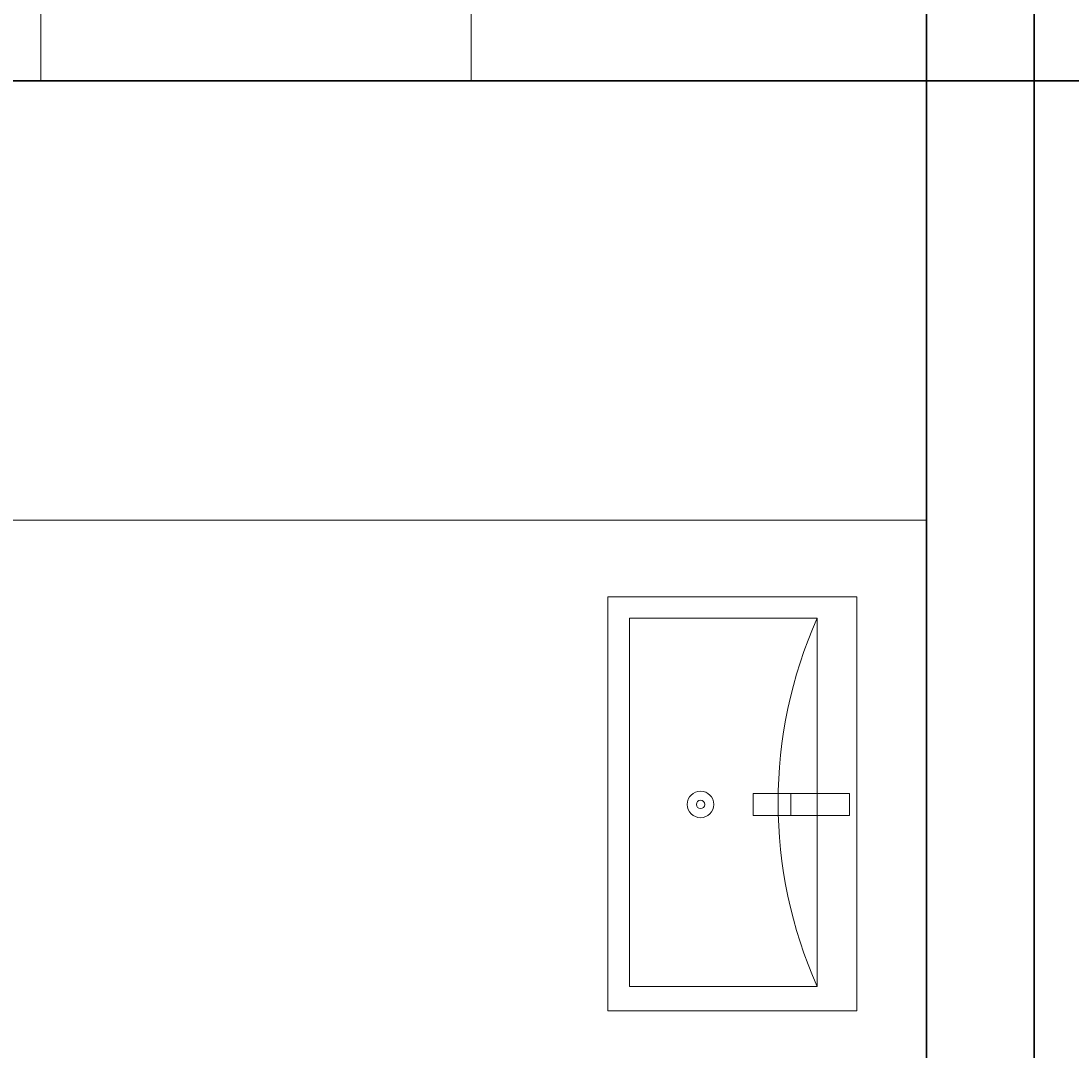
# Model space of a CAD drawing. Units: inches. Extents: x -61 to 1599, y -1316 to 257.
# Tile 71 of 204: x 347 to 406, y -680 to -623. Entities that reach past the tile are written whole.
import ezdxf

# ---------------------------------------------------------------- set-up
doc = ezdxf.new("R2010")
doc.units = ezdxf.units.IN
doc.header["$MEASUREMENT"] = 0
for name, color, linetype, lineweight in [('A-ANNO-DIMS', 2, 'Continuous', 18), ('A-FLOR-FIXT', 8, 'Continuous', 18), ('WALLS', 4, 'Continuous', 35), ('WINDOWS', 220, 'Continuous', 18)]:
    doc.layers.add(name, color=color, linetype=linetype, lineweight=lineweight)
doc.styles.get("Standard").update_dxf_attribs({"font": 'arial.ttf'})
doc.dimstyles.get("Standard").update_dxf_attribs({"dimtxt": 0.18, "dimasz": 0.18, "dimexe": 0.18, "dimexo": 0.0625, "dimgap": 0.09, "dimtad": 0, "dimtih": 1, "dimtoh": 1, "dimdec": 0, "dimzin": 0, "dimdsep": 46, "dimlunit": 3, "dimtxsty": 'Standard', "dimcen": 0.09, "dimadec": 0, "dimazin": 0, "dimtfac": 1, "dimtdec": 0, "dimtofl": 0, "dimtmove": 0, "dimatfit": 3, "dimfxl": 1, "dimtolj": 1, "dimtzin": 0, "dimarcsym": 0})

# ---------------------------------------------------------------- blocks, each defined once
blk = doc.blocks.new('WIN-24IN')
for p, q in [((0, 4.5), (0, 9)), ((0, 9), (0, 0)), ((24, 9), (24, 0)), ((0, 5.192), (24, 5.192)), ((0, 4.5), (24, 4.5))]:
    blk.add_line(p, q)
blk = doc.blocks.new('LAVATORY-WALL')
blk.add_line((10.191, 12.111), (10.191, 10.884))
for points in [[(13.866, 0), (0, 0), (0, 23.069), (13.866, 23.069)], [(13.866, 0), (0, 0), (0, 23.069), (13.866, 23.069)], [(1.203, 1.342), (1.203, 21.884), (11.667, 21.884), (11.667, 1.342)], [(8.089, 10.884), (8.089, 12.111), (13.47, 12.111), (13.47, 10.884)]]:
    blk.add_lwpolyline(points, close=True)
for radius in [0.74, 0.233]:
    blk.add_circle((5.161, 11.497), radius)
blk.add_arc((34.73, 11.613), 25.246, 155.99389, 204.00611)
blk = doc.blocks.new('*D710')
at = {"layer": 'A-ANNO-DIMS', "color": 0, "lineweight": -2, "transparency": 16777216}
for p, q in [((319.703, -465.385), (319.703, -1315.725)), ((403.703, -465.385), (403.703, -1315.725)), ((319.883, -1315.545), (361.484, -1315.545)), ((403.523, -1315.545), (361.921, -1315.545))]:
    blk.add_line(p, q, dxfattribs=at)
at = {"layer": 'A-ANNO-DIMS', "color": 0, "transparency": 16777216}
for points in [[(319.883, -1315.515), (319.883, -1315.575), (319.703, -1315.545)], [(403.523, -1315.515), (403.523, -1315.575), (403.703, -1315.545)]]:
    blk.add_solid(points, dxfattribs=at)
at = {"layer": 'DEFPOINTS', "color": 0, "transparency": 16777216}
for p in [(319.703, -465.323), (403.703, -465.323), (403.703, -1315.545)]:
    blk.add_point(p, dxfattribs=at)
at = {"layer": 'A-ANNO-DIMS', "color": 0, "transparency": 16777216, "insert": (361.703, -1315.545), "char_height": 0.18, "attachment_point": 5}
blk.add_mtext('\\A1;84', dxfattribs=at)

msp = doc.modelspace()

# ---------------------------------------------------------------- linework, layer by layer
at = {"layer": 'A-FLOR-FIXT'}
msp.add_line((327.7028, -650.414), (397.7028, -650.414), dxfattribs=at)
at = {"layer": 'WALLS'}
for p, q in [((397.7028, -616.9446), (397.7028, -733.9446)), ((403.7028, -616.9446), (403.7028, -733.9446)), ((327.7028, -625.9446), (397.7028, -625.9446)), ((397.7028, -625.9446), (403.7028, -625.9446)), ((403.7028, -625.9446), (535.7028, -625.9446))]:
    msp.add_line(p, q, dxfattribs=at)

# ---------------------------------------------------------------- block references
at = {"layer": 'A-FLOR-FIXT'}
msp.add_blockref('LAVATORY-WALL', (379.936, -677.7577), dxfattribs=at)
at = {"layer": 'WINDOWS'}
msp.add_blockref('WIN-24IN', (348.3196, -625.9447), dxfattribs=at)

# ---------------------------------------------------------------- dimensions: what is measured, and where the dimension line sits
at = {"layer": 'A-ANNO-DIMS'}
dim = msp.add_linear_dim(base=(403.7028, -1315.5446), p1=(319.7028, -465.3229), p2=(403.7028, -465.3229), dimstyle='Standard', override={"dimdec": 0, "dimlfac": 1, "dimrnd": 0, "dimzin": 0, "dimdsep": 46, "dimlunit": 2}, dxfattribs=at)
dim.commit()
dim.dimension.update_dxf_attribs({"geometry": '*D710', "text_midpoint": (361.7028, -1315.5446)})

doc.saveas('drawing.dxf')
